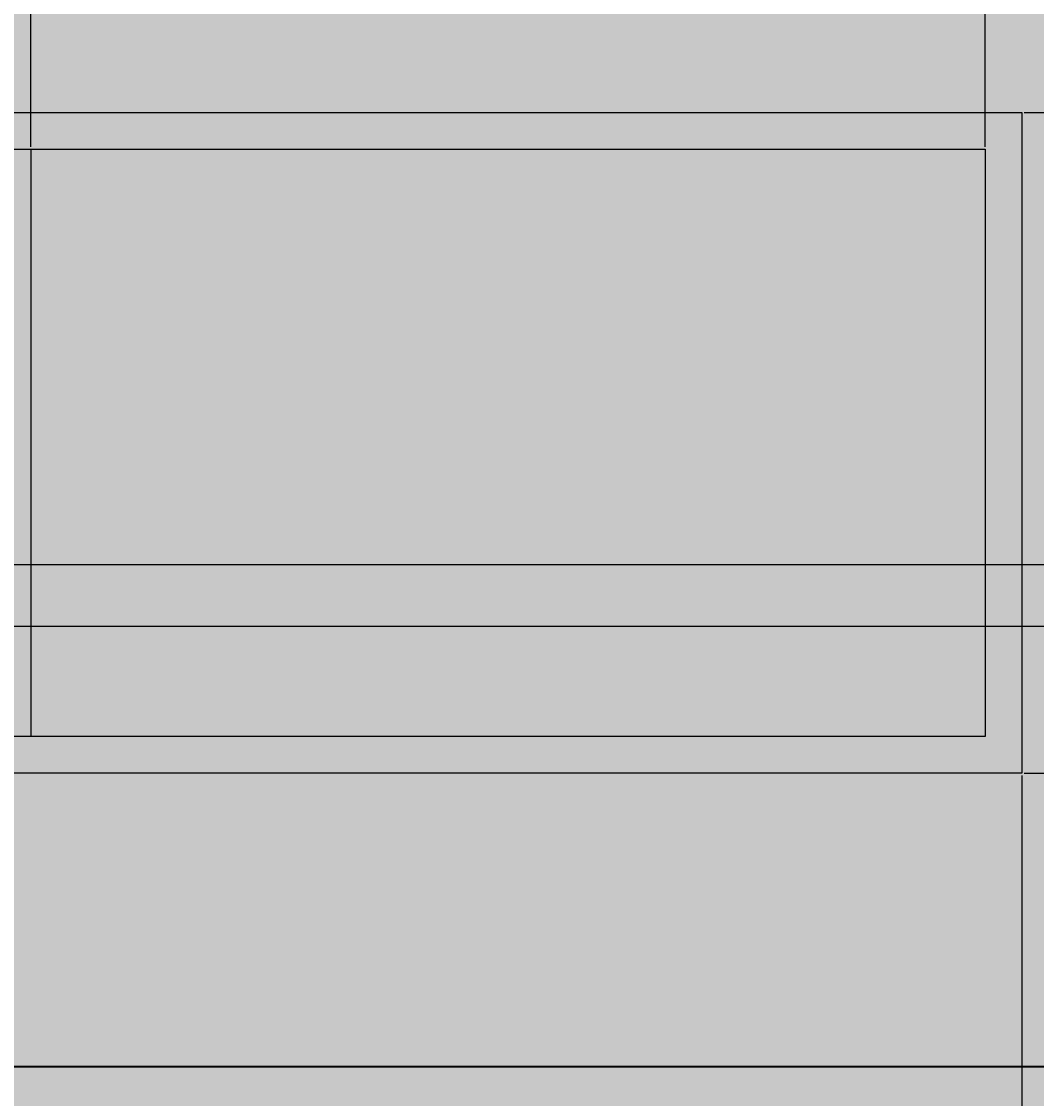
# Model space of a CAD drawing. Units: inches. Extents: x 4508 to 4723, y 847 to 1020.
# Tile 19 of 32: x 4631 to 4658, y 878 to 907. Entities that reach past the tile are written whole.
import ezdxf

# ---------------------------------------------------------------- set-up
doc = ezdxf.new("R2010")
doc.units = ezdxf.units.IN
for name, color, linetype, lineweight in [('A-ANNO-DIMS', 2, 'Continuous', 18), ('A-FURN', 8, 'Continuous', 25), ('A-WALL', 7, 'Continuous', 35), ('A-WALL-PATT', 254, 'Continuous', 13)]:
    doc.layers.add(name, color=color, linetype=linetype, lineweight=lineweight)
doc.styles.get("Standard").update_dxf_attribs({"font": 'arial.ttf'})
doc.dimstyles.get("Standard").update_dxf_attribs({"dimtxt": 0.18, "dimasz": 0.18, "dimexe": 0.18, "dimexo": 0.0625, "dimgap": 0.09, "dimtad": 0, "dimtih": 1, "dimtoh": 1, "dimdec": 4, "dimzin": 0, "dimdsep": 46, "dimtxsty": 'Standard', "dimcen": 0.09, "dimadec": 0, "dimazin": 0, "dimtfac": 1, "dimtdec": 4, "dimtofl": 0, "dimtmove": 0, "dimatfit": 3, "dimfxl": 1, "dimtolj": 1, "dimtzin": 0, "dimarcsym": 0})

# ---------------------------------------------------------------- blocks, each defined once
blk = doc.blocks.new('*D24')
at = {"layer": 'A-ANNO-DIMS', "color": 0, "lineweight": -2, "transparency": 16777216}
for p, q in [((4549.994, 886.684), (4549.994, 866.617)), ((4657.994, 886.684), (4657.994, 866.617)), ((4550.174, 866.797), (4603.713, 866.797)), ((4657.814, 866.797), (4604.274, 866.797))]:
    blk.add_line(p, q, dxfattribs=at)
at = {"layer": 'A-ANNO-DIMS', "color": 0, "lineweight": 9, "transparency": 16777216}
for points in [[(4550.174, 866.827), (4550.174, 866.767), (4549.994, 866.797)], [(4657.814, 866.827), (4657.814, 866.767), (4657.994, 866.797)]]:
    blk.add_solid(points, dxfattribs=at)
at = {"layer": 'Defpoints', "color": 0, "lineweight": 9, "transparency": 16777216}
for p in [(4549.994, 886.747), (4657.994, 886.747), (4657.994, 866.797)]:
    blk.add_point(p, dxfattribs=at)
at = {"layer": 'A-ANNO-DIMS', "color": 0, "transparency": 16777216, "insert": (4603.994, 866.797), "char_height": 0.18, "attachment_point": 5}
blk.add_mtext('\\A1;108', dxfattribs=at)
blk = doc.blocks.new('*D25')
at = {"layer": 'A-ANNO-DIMS', "color": 0, "lineweight": -2, "transparency": 16777216}
for p, q in [((4658.056, 904.747), (4702.124, 904.747)), ((4701.944, 904.567), (4701.944, 895.929)), ((4701.944, 886.927), (4701.944, 895.565)), ((4658.056, 886.747), (4702.124, 886.747))]:
    blk.add_line(p, q, dxfattribs=at)
at = {"layer": 'A-ANNO-DIMS', "color": 0, "lineweight": 9, "transparency": 16777216}
for points in [[(4701.914, 904.567), (4701.974, 904.567), (4701.944, 904.747)], [(4701.914, 886.927), (4701.974, 886.927), (4701.944, 886.747)]]:
    blk.add_solid(points, dxfattribs=at)
at = {"layer": 'Defpoints', "color": 0, "lineweight": 9, "transparency": 16777216}
for p in [(4657.994, 904.747), (4701.944, 904.747), (4657.994, 886.747)]:
    blk.add_point(p, dxfattribs=at)
at = {"layer": 'A-ANNO-DIMS', "color": 0, "transparency": 16777216, "insert": (4701.944, 895.747), "char_height": 0.18, "attachment_point": 5}
blk.add_mtext('\\A1;18', dxfattribs=at)
blk = doc.blocks.new('*D31')
at = {"layer": 'A-ANNO-DIMS', "color": 0, "lineweight": -2, "transparency": 16777216}
for p, q in [((4630.994, 903.809), (4630.994, 1002.877)), ((4631.174, 1002.697), (4643.773, 1002.697)), ((4656.814, 1002.697), (4644.214, 1002.697)), ((4656.994, 903.809), (4656.994, 1002.877))]:
    blk.add_line(p, q, dxfattribs=at)
at = {"layer": 'A-ANNO-DIMS', "color": 0, "lineweight": 9, "transparency": 16777216}
for points in [[(4631.174, 1002.727), (4631.174, 1002.667), (4630.994, 1002.697)], [(4656.814, 1002.727), (4656.814, 1002.667), (4656.994, 1002.697)]]:
    blk.add_solid(points, dxfattribs=at)
at = {"layer": 'Defpoints', "color": 0, "lineweight": 9, "transparency": 16777216}
for p in [(4656.994, 1002.697), (4630.994, 903.747), (4656.994, 903.747)]:
    blk.add_point(p, dxfattribs=at)
at = {"layer": 'A-ANNO-DIMS', "color": 0, "transparency": 16777216, "insert": (4643.994, 1002.697), "char_height": 0.18, "attachment_point": 5}
blk.add_mtext('\\A1;26', dxfattribs=at)
blk = doc.blocks.new('*D35')
at = {"layer": 'A-ANNO-DIMS', "color": 0, "lineweight": -2, "transparency": 16777216}
for p, q in [((4625.361, 892.428), (4702.124, 892.428)), ((4701.944, 892.248), (4701.944, 891.769)), ((4701.944, 890.927), (4701.944, 891.405)), ((4625.361, 890.747), (4702.124, 890.747))]:
    blk.add_line(p, q, dxfattribs=at)
at = {"layer": 'A-ANNO-DIMS', "color": 0, "lineweight": 9, "transparency": 16777216}
for points in [[(4701.914, 892.248), (4701.974, 892.248), (4701.944, 892.428)], [(4701.914, 890.927), (4701.974, 890.927), (4701.944, 890.747)]]:
    blk.add_solid(points, dxfattribs=at)
at = {"layer": 'Defpoints', "color": 0, "lineweight": 9, "transparency": 16777216}
for p in [(4625.298, 892.428), (4701.944, 892.428), (4625.298, 890.747)]:
    blk.add_point(p, dxfattribs=at)
at = {"layer": 'A-ANNO-DIMS', "color": 0, "transparency": 16777216, "insert": (4701.944, 891.587), "char_height": 0.18, "attachment_point": 5}
blk.add_mtext('\\A1;1.681', dxfattribs=at)

msp = doc.modelspace()

# ---------------------------------------------------------------- hatches: boundary and pattern name
at = {"layer": 'A-WALL-PATT', "transparency": 33554508}
h = msp.add_hatch(color=256, dxfattribs=at)
h.dxf.hatch_style = 1
h.paths.add_polyline_path([(4661.6706, 954.043, -0.3739004), (4658.5765, 957.6021, -1), (4665.7646, 957.6021, -0.3739004), (4662.6706, 954.043), (4662.6706, 944.4021, -0.2114781), (4670.3062, 945.0869), (4670.3062, 968.0592, -0.4632086), (4663.3246, 973.9783, -0.4632086), (4670.3062, 979.8975), (4670.3062, 994.7469), (4588.9938, 994.7469), (4588.9938, 904.7469), (4657.9938, 904.7469), (4657.9938, 886.7469), (4549.9938, 886.7469), (4549.9938, 878.7469), (4693.9938, 878.7469), (4693.9938, 994.7469), (4671.8062, 994.7469), (4671.8062, 979.4411, -0.2941682), (4675.3246, 973.9783, -0.2941682), (4671.8062, 968.5156), (4671.8062, 944.4278, -0.2741114), (4676.7298, 936.1217, -0.2741114), (4671.8062, 927.8155), (4671.8062, 907.6998, -0.3779645), (4677.0562, 901.7469, -0.3779645), (4671.8062, 895.7939), (4671.8062, 883.7469), (4670.3062, 883.7469), (4670.3062, 895.7939, -0.3779645), (4665.0562, 901.7469, -0.3779645), (4670.3062, 907.6998), (4670.3062, 927.1564, -0.2114781), (4662.6706, 927.8412), (4662.6706, 918.2003, -0.3739004), (4665.7646, 914.6412, -1), (4658.5765, 914.6412, -0.3739004), (4661.6706, 918.2003), (4661.6706, 928.4807, -0.2391825), (4657.7936, 936.1217, -0.2391825), (4661.6706, 943.7626)])
at = {"layer": 'A-WALL-PATT', "transparency": 33554681}
h = msp.add_hatch(color=256, dxfattribs=at)
h.dxf.hatch_style = 1
h.paths.add_polyline_path([(4577.4938, 903.7469), (4550.9938, 903.7469), (4550.9938, 887.7469), (4577.4938, 887.7469)], flags=0)
h.paths.add_polyline_path([(4603.9938, 903.7469), (4577.9938, 903.7469), (4577.9938, 887.7469), (4603.9938, 887.7469)], flags=0)
h.paths.add_polyline_path([(4656.9938, 903.7469), (4630.9938, 903.7469), (4630.9938, 887.7469), (4656.9938, 887.7469)], flags=0)
h.paths.add_polyline_path([(4657.9938, 904.7469), (4549.9938, 904.7469), (4549.9938, 886.7469), (4657.9938, 886.7469)])
h.paths.add_polyline_path([(4656.9938, 903.7469), (4656.9938, 887.7469), (4550.9938, 887.7469), (4550.9938, 903.7469)], flags=16)
h = msp.add_hatch(color=256, dxfattribs=at)
h.dxf.hatch_style = 1
h.paths.add_polyline_path([(4577.4938, 903.7469), (4550.9938, 903.7469), (4550.9938, 887.7469), (4577.4938, 887.7469)])
h.paths.add_polyline_path([(4603.9938, 903.7469), (4577.9938, 903.7469), (4577.9938, 887.7469), (4603.9938, 887.7469)])
h.paths.add_polyline_path([(4656.9938, 903.7469), (4630.9938, 903.7469), (4630.9938, 887.7469), (4656.9938, 887.7469)])
h = msp.add_hatch(color=256, dxfattribs=at)
h.dxf.hatch_style = 1
h.paths.add_polyline_path([(4604.4938, 903.7469), (4603.9938, 903.7469), (4603.9938, 887.7469), (4604.4938, 887.7469)])
h.paths.add_polyline_path([(4630.9938, 903.7469), (4630.4938, 903.7469), (4630.4938, 887.7469), (4630.9938, 887.7469)])
h.paths.add_polyline_path([(4577.9938, 903.7469), (4577.4938, 903.7469), (4577.4938, 887.7469), (4577.9938, 887.7469)])
at = {"layer": 'A-WALL-PATT', "transparency": 33554556}
h = msp.add_hatch(color=256, dxfattribs=at)
h.dxf.hatch_style = 1
h.paths.add_polyline_path([(4689.9938, 878.7469), (4549.9938, 878.7469), (4549.9938, 874.7469), (4689.9938, 874.7469)])

# ---------------------------------------------------------------- linework, layer by layer
at = {"layer": 'A-FURN'}
msp.add_line((4630.9938, 903.7469), (4630.9938, 887.7469), dxfattribs=at)
for points in [[(4657.9938, 886.7469), (4549.9938, 886.7469), (4549.9938, 904.7469), (4657.9938, 904.7469)], [(4656.9938, 887.7469), (4550.9938, 887.7469), (4550.9938, 903.7469), (4656.9938, 903.7469)]]:
    msp.add_lwpolyline(points, close=True, dxfattribs=at)
at = {"layer": 'A-WALL'}
msp.add_line((4693.9938, 878.7469), (4549.9938, 878.7469), dxfattribs=at)

# ---------------------------------------------------------------- dimensions: what is measured, and where the dimension line sits
at = {"layer": 'A-ANNO-DIMS'}
for base, p1, p2, picture, middle in [((4656.9938, 1002.6969), (4630.9938, 903.7469), (4656.9938, 903.7469), '*D31', (4643.9938, 1002.6969)), ((4657.9938, 866.7969), (4549.9938, 886.7469), (4657.9938, 886.7469), '*D24', (4603.9938, 866.7969))]:
    dim = msp.add_linear_dim(base=base, p1=p1, p2=p2, dimstyle='Standard', override={"dimdec": 0, "dimlfac": 1, "dimrnd": 0, "dimzin": 0, "dimdsep": 46, "dimlunit": 2}, dxfattribs=at)
    dim.commit()
    dim.dimension.update_dxf_attribs({"geometry": picture, "text_midpoint": middle})
for base, p1, p2, override, picture, middle in [((4701.9438, 904.7469), (4657.9938, 886.7469), (4657.9938, 904.7469), {"dimdec": 0, "dimlfac": 1, "dimrnd": 0, "dimzin": 0, "dimdsep": 46, "dimlunit": 2}, '*D25', (4701.9438, 895.7469)), ((4701.9438, 892.4277), (4625.2983, 890.7469), (4625.2983, 892.4277), {"dimdec": 3, "dimlfac": 1, "dimrnd": 0, "dimzin": 0, "dimdsep": 46, "dimlunit": 2}, '*D35', (4701.9438, 891.5873))]:
    dim = msp.add_linear_dim(base=base, p1=p1, p2=p2, angle=90, dimstyle='Standard', override=override, dxfattribs=at)
    dim.commit()
    dim.dimension.update_dxf_attribs({"geometry": picture, "text_midpoint": middle})

doc.saveas('drawing.dxf')
